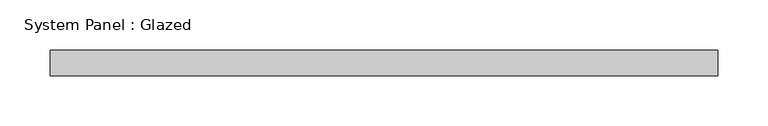
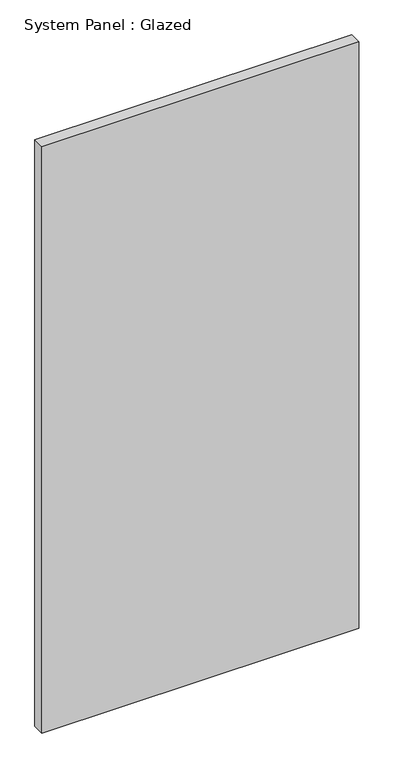
"""IFC4 building model written with IfcOpenShell, lengths in millimetres: plate geometry, System Panel : Glazed."""

from ifc_helpers import new_model, si_unit, origin, origin_with_axes, place, context, project, spatial, polyline, outline, extrude, source, transform, mapped, element, save


def system_panel_glazed_3378ba69(model_context):
    return source(origin(), model_context, "Body", "SweptSolid", [
        extrude(outline(polyline([(333.375, 19.05), (-333.375, 19.05), (-333.375, 44.45), (333.375, 44.45), (333.375, 19.05)])), origin_with_axes(), (0.0, 0.0, 1.0), 1304.1740318),
    ])


if __name__ == "__main__":
    model = new_model("IFC4")
    model_context = context("Model", 3, world=origin())
    ifc_project = project(units=[si_unit("LENGTHUNIT", "METRE", prefix="MILLI")], contexts=[model_context])
    site = spatial("IfcSite", under=ifc_project)
    building = spatial("IfcBuilding", under=site)
    placement = place(None, origin())
    system_panel_glazed_shape = system_panel_glazed_3378ba69(model_context)
    element("IfcPlate", 1, ObjectType="System Panel : Glazed", at=placement, inside=building, context=model_context, shape_type="MappedRepresentation", body=[
        mapped(system_panel_glazed_shape, transform((0.0, 0.0, 0.0), x_axis=(1.0, 0.0, 0.0), y_axis=(0.0, 1.0, 0.0), z_axis=(0.0, 0.0, 1.0))),
    ])
    save(model, "model.ifc")

# Revit data of these elements
# Type "System Panel : Glazed"
#   Construction Type Id = "GSP4R"
#   Analytic Construction = "1/8 in Pilkington single glazing"
#   Visual Light Transmittance = 0.9
#   Solar Heat Gain Coefficient = 0.86
#   Heat Transfer Coefficient (U) = 1.18115 BTU/(h·ft²·°F)
#   Define Thermal Properties by = 1
# Element 1 (IfcPlate, "System Panel : Glazed")
#   Materials on its faces: "Glass"
# Materials
#   "Glass": class "Glass", colour RGB 0 128 192, transparency 0.75, Description = "Soda Lime Glass", Cost = 0
